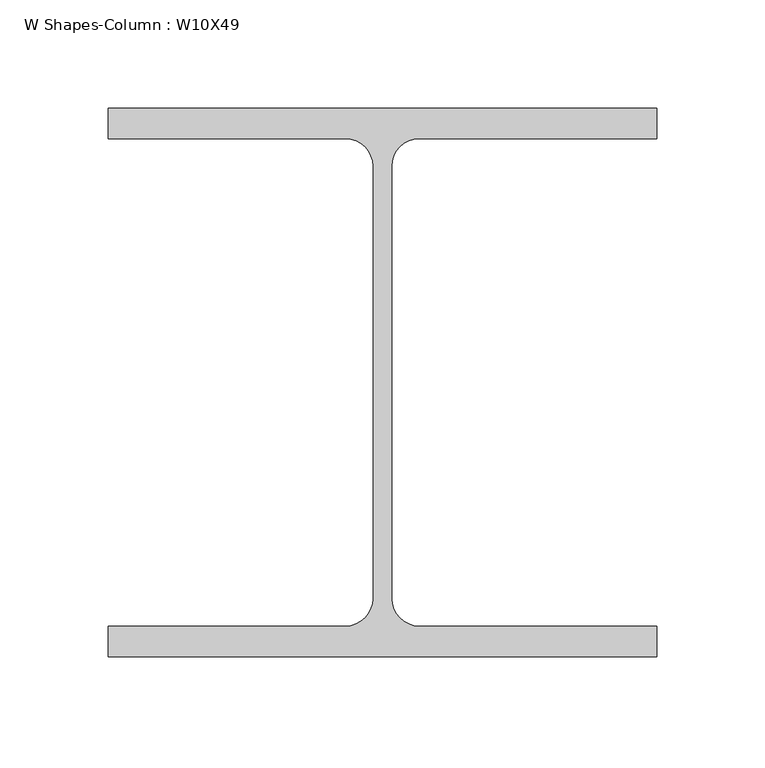
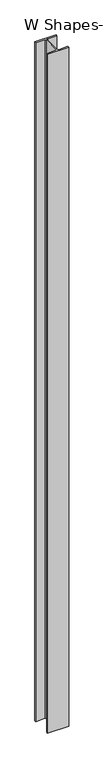
"""IFC4 building model written with IfcOpenShell, lengths in millimetres: column geometry, W Shapes-Column : W10X49."""

from ifc_helpers import new_model, si_unit, point, frame, frame_2d, origin, place, context, project, spatial, polyline, circle_curve, trimmed, segment, composite_curve, outline, extrude, source, transform, mapped, element, save


def w_shapes_column_w10x49_3bdde7d6(model_context):
    return source(origin(), model_context, "Body", "SweptSolid", [
        extrude(outline(composite_curve([segment(polyline([(127.0, 127.0), (127.0, 112.776), (17.018, 112.776)]), True, "CONTINUOUS"), segment(trimmed(circle_curve(frame_2d((17.018, 100.076)), 12.7), [point((17.018, 112.776))], [point((4.318, 100.076))], True, "CARTESIAN"), True, "CONTINUOUS"), segment(polyline([(4.318, 100.076), (4.318, -100.076)]), True, "CONTINUOUS"), segment(trimmed(circle_curve(frame_2d((17.018, -100.076)), 12.7), [point((4.318, -100.076))], [point((17.018, -112.776))], True, "CARTESIAN"), True, "CONTINUOUS"), segment(polyline([(17.018, -112.776), (127.0, -112.776), (127.0, -127.0), (-127.0, -127.0), (-127.0, -112.776), (-17.018, -112.776)]), True, "CONTINUOUS"), segment(trimmed(circle_curve(frame_2d((-17.018, -100.076)), 12.7), [point((-17.018, -112.776))], [point((-4.318, -100.076))], True, "CARTESIAN"), True, "CONTINUOUS"), segment(polyline([(-4.318, -100.076), (-4.318, 100.076)]), True, "CONTINUOUS"), segment(trimmed(circle_curve(frame_2d((-17.018, 100.076)), 12.7), [point((-4.318, 100.076))], [point((-17.018, 112.776))], True, "CARTESIAN"), True, "CONTINUOUS"), segment(polyline([(-17.018, 112.776), (-127.0, 112.776), (-127.0, 127.0), (127.0, 127.0)]), True, "CONTINUOUS")], self_intersect=False)), frame((0.0, 0.0, -2133.5), z_axis=(0.0, 0.0, 1.0), x_axis=(1.0, 0.0, 0.0)), (0.0, 0.0, 1.0), 8534.0),
    ])


if __name__ == "__main__":
    model = new_model("IFC4")
    model_context = context("Model", 3, world=origin())
    ifc_project = project(units=[si_unit("LENGTHUNIT", "METRE", prefix="MILLI")], contexts=[model_context])
    site = spatial("IfcSite", under=ifc_project)
    building = spatial("IfcBuilding", under=site)
    placement = place(None, origin())
    w_shapes_column_w10x49_shape = w_shapes_column_w10x49_3bdde7d6(model_context)
    element("IfcColumn", 1, ObjectType="W Shapes-Column : W10X49", at=placement, inside=building, context=model_context, shape_type="MappedRepresentation", body=[
        mapped(w_shapes_column_w10x49_shape, transform((0.0, 0.0, 0.0), x_axis=(1.0, 0.0, 0.0), y_axis=(0.0, 1.0, 0.0), z_axis=(0.0, 0.0, 1.0))),
    ])
    save(model, "model.ifc")

# Revit data of these elements
# Type "W Shapes-Column : W10X49"
#   Section Name Key = "W10X49"
#   Width = 10.000"
#   Web Thickness = 0.340"
#   Web Fillet = 0.500"
#   Warping Constant = 2070.00 in⁶
#   Torsional Moment of Inertia = 1.39 in⁴
#   Section Area = 14.40 in²
#   Plastic Modulus weak axis = 28.30 in³
#   Plastic Modulus strong axis = 60.40 in³
#   Perimeter = 4.875 ft²/ft
#   Nominal Weight = 49.00 lbf/ft
#   Moment of Inertia weak axis = 93.40 in⁴
#   Moment of Inertia strong axis = 272.00 in⁴
#   Height = 10.000"
#   Flange Thickness = 0.560"
#   Elastic Modulus weak axis = 18.70 in³
#   Elastic Modulus strong axis = 54.60 in³
#   Clear Web Height = 0' - 7 1/2"
#   Centroid Vertical = 5.000"
#   Centroid Horizontal = 5.000"
#   Bolt Spacing = 0' - 5 1/2"
#   Structural Material [instance default] = Steel ASTM A992
#   Principal Axes Angle = 0
# Element 1 (IfcColumn, "W Shapes-Column : W10X49")
#   Materials on its faces: "Steel ASTM A992"
# Materials
#   "Steel ASTM A992": class "Metal", colour RGB 199 199 199, transparency 0, Description = "Structural steel 50ksi", Cost = 0
